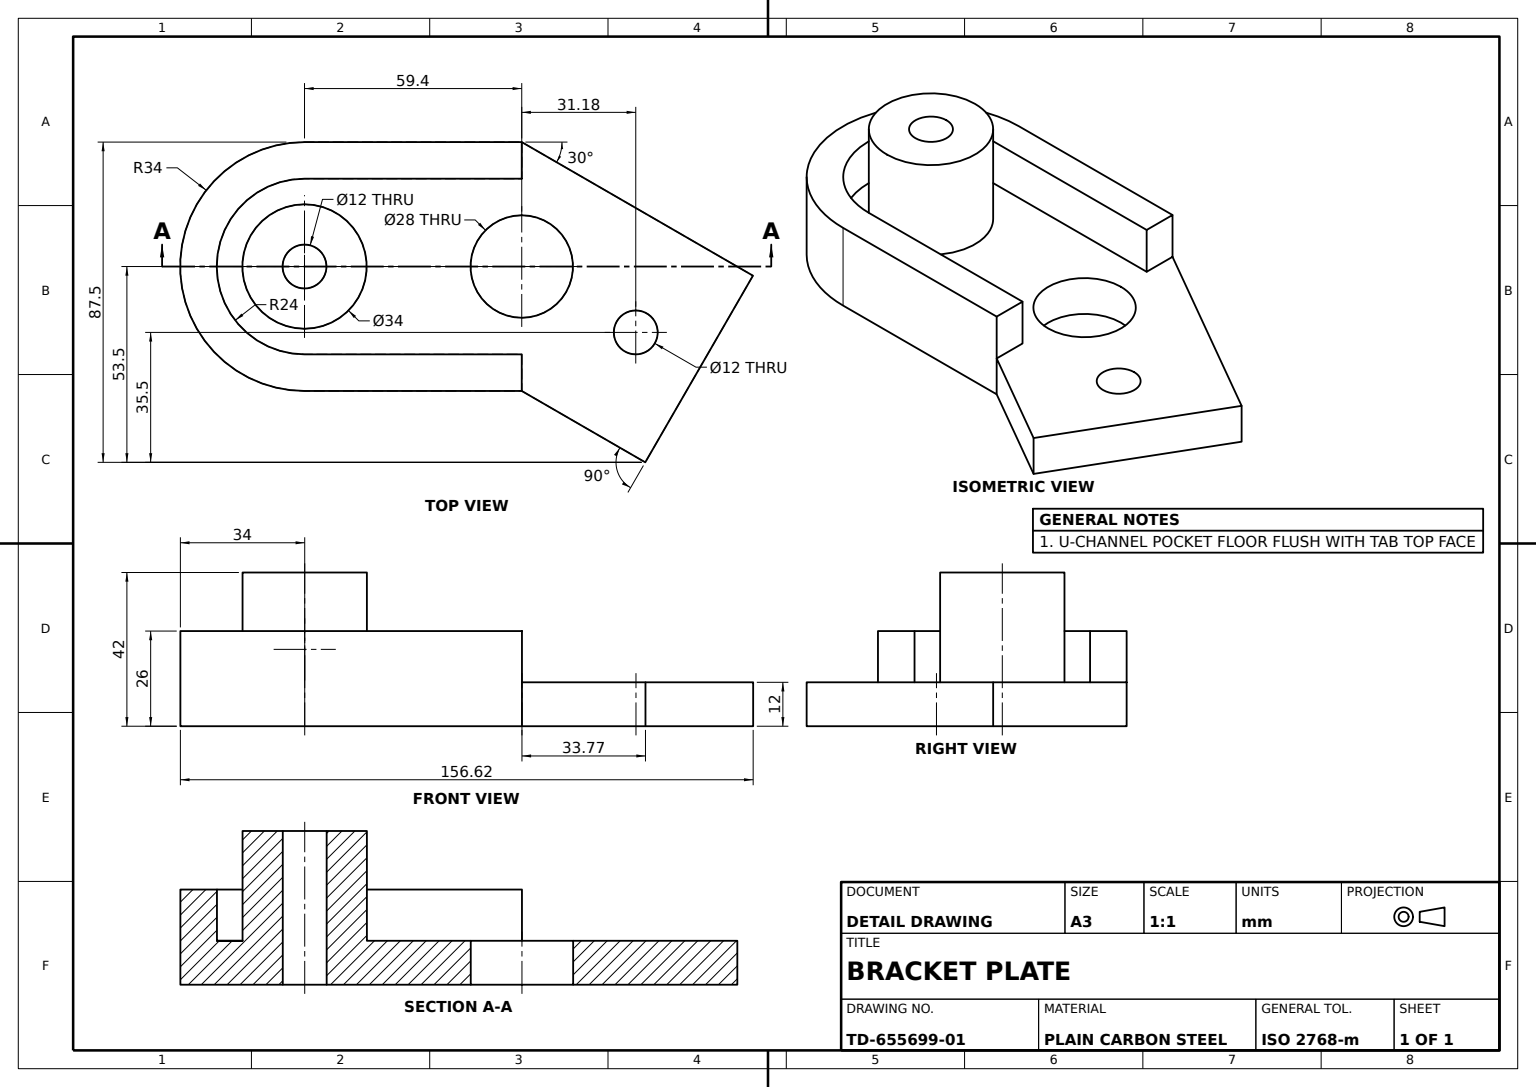
SolidWorks part; units mm, degrees
material "Plain Carbon Steel"
ref_plane "Front Plane" through (0, 0, 0) normal (0, 0, 1) x (1, 0, 0)
ref_plane "Top Plane" through (0, 0, 0) normal (0, 1, 0) x (1, 0, 0)
ref_plane "Right Plane" through (0, 0, 0) normal (1, 0, 0) x (0, 0, -1)
sketch "Base Profile Sketch" plane through (0, 0, 0) normal (0, 1, 0) x (1, 0, 0)
  line L0 (0, 34) -> (59.4, 34)
  line L1 (59.4, 34) -> (59.4, -34)
  line L2 (59.4, -34) -> (0, -34)
  arc A0 (0, 34) -> (0, -34) centre (0, 0) ccw
  dimension "D1" = 68
  dimension "D2" = 59.4
extrude "Base Plate" add sketch "Base Profile Sketch" along normal blind 26
sketch "Pocket Profile Sketch" plane through (0, 26, 0) normal (0, 1, 0) x (1, 0, 0)
  line L0 (0, 24) -> (59.4, 24)
  line L1 (59.4, -34) -> (59.4, 34) construction
  line L2 (59.4, 24) -> (59.4, -24)
  line L3 (59.4, -24) -> (0, -24)
  arc A0 (0, 24) -> (0, -24) centre (0, 0) ccw
  dimension "D1" = 48
extrude "U Pocket 14 Deep" cut sketch "Pocket Profile Sketch" against normal blind 14
sketch "Angled Tab Sketch" plane through (0, 12, 0) normal (0, 1, 0) x (1, 0, 0)
  line L0 (59.4, 0) -> (78.6368, 0) construction
  line L1 (59.4, -24) -> (59.4, 24) construction
  line L2 (59.4, 34) -> (122.6199, -2.5)
  line L3 (59.4, 0) -> (110.912, -29.7405) construction
  line L4 (122.6199, -2.5) -> (93.175, -53.5)
  line L5 (59.4, -34) -> (93.175, -53.5)
  line L6 (59.4, 34) -> (59.4, -34)
  dimension "D1" = 30
  dimension "D2" = 56
extrude "Angled Tab 30deg" add sketch "Angled Tab Sketch" against normal blind 12
sketch "Boss Circle Sketch" plane through (0, 12, 0) normal (0, 1, 0) x (1, 0, 0)
  circle A0 centre (0, 0) radius 17
  dimension "D1" = 34
extrude "Boss Ø34" add sketch "Boss Circle Sketch" along normal blind 30
sketch "Boss Bore Sketch" plane through (0, 42, 0) normal (0, 1, 0) x (1, 0, 0)
  circle A0 centre (0, 0) radius 6
  dimension "D1" = 12
extrude "Boss Bore Ø12" cut sketch "Boss Bore Sketch" against normal through all
sketch "Tab Holes Sketch" plane through (0, 12, 0) normal (0, 1, 0) x (1, 0, 0)
  line L1 (59.4, 0) -> (107.8974, -28) construction
  line L2 (93.175, -53.5) -> (122.6199, -2.5) construction
  circle A0 centre (59.4, 0) radius 14
  circle A1 centre (90.5769, -18) radius 6
  dimension "D1" = 28
  dimension "D2" = 12
  dimension "D3" = 36
extrude "Tab Holes Ø28 and Ø12" cut sketch "Tab Holes Sketch" against normal blind 30
